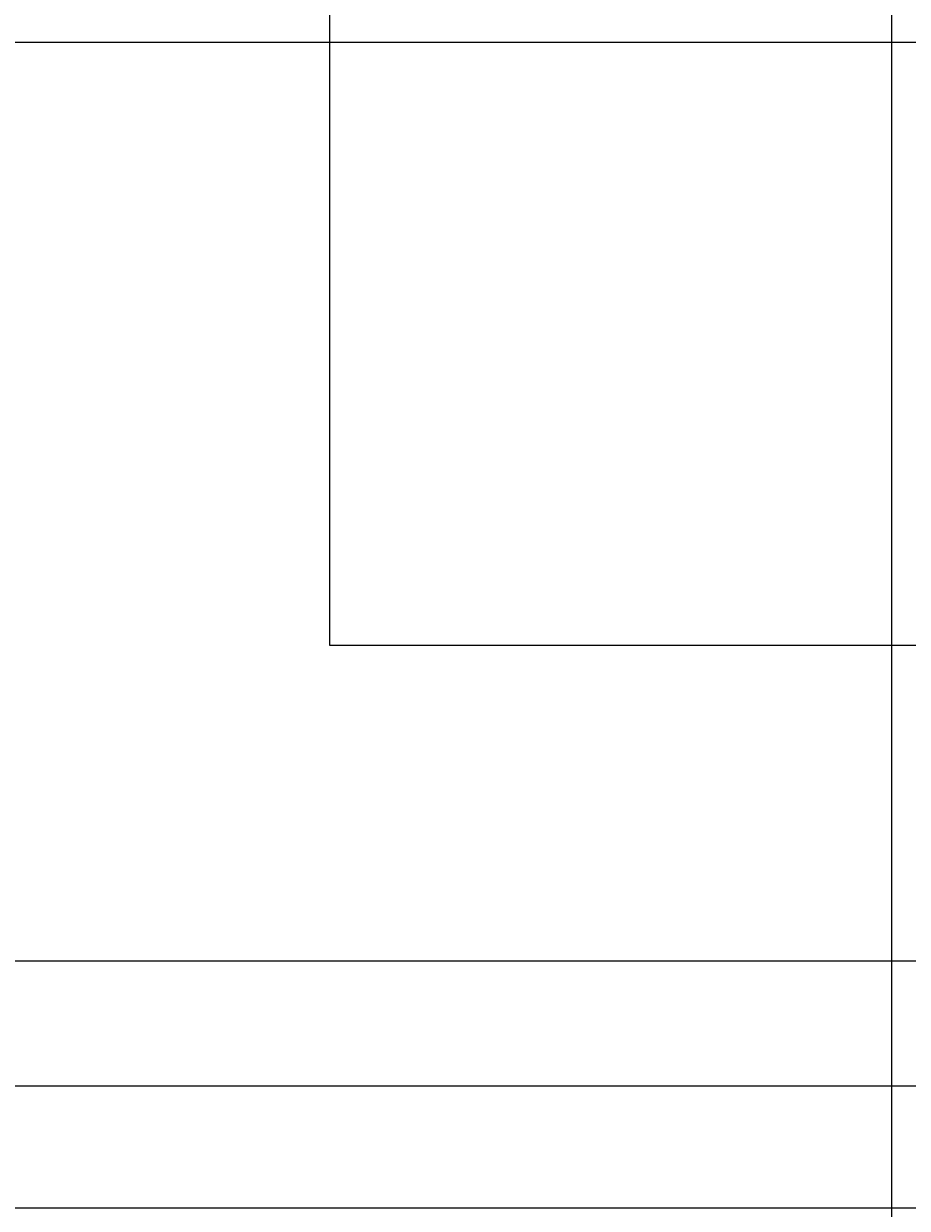
# Model space of a CAD drawing. Units: inches. Extents: x 35362 to 73946, y 43607 to 67532.
# Tile 87 of 134: x 51337 to 51924, y 47544 to 48331. Entities that reach past the tile are written whole.
import ezdxf

# ---------------------------------------------------------------- set-up
doc = ezdxf.new("R2010")
doc.units = ezdxf.units.IN
doc.header["$MEASUREMENT"] = 0
doc.layers.add('A-ANNO-DIMS', color=2, linetype='Continuous', lineweight=18)
doc.layers.add('E-WIRE', color=3, linetype='Continuous', lineweight=25)
doc.styles.get("Standard").update_dxf_attribs({"font": 'arial.ttf'})
doc.dimstyles.get("Standard").update_dxf_attribs({"dimtxt": 0.18, "dimasz": 0.18, "dimexe": 0.18, "dimexo": 0.0625, "dimgap": 0.09, "dimtad": 0, "dimtih": 1, "dimtoh": 1, "dimdec": 4, "dimzin": 0, "dimdsep": 46, "dimtxsty": 'Standard', "dimcen": 0.09, "dimadec": 0, "dimazin": 0, "dimtfac": 1, "dimtdec": 4, "dimtofl": 0, "dimtmove": 0, "dimatfit": 3, "dimfxl": 1, "dimtolj": 1, "dimtzin": 0, "dimarcsym": 0})

# ---------------------------------------------------------------- blocks, each defined once
blk = doc.blocks.new('*D11')
at = {"layer": 'A-ANNO-DIMS', "color": 0, "lineweight": -2, "transparency": 16777216}
for p, q in [((47978.66, 56028.77), (47978.66, 43606.68)), ((53109.76, 56028.77), (53109.76, 43606.68)), ((47978.84, 43606.86), (50543.87, 43606.86)), ((53109.58, 43606.86), (50544.55, 43606.86))]:
    blk.add_line(p, q, dxfattribs=at)
at = {"layer": 'A-ANNO-DIMS', "color": 0, "transparency": 16777216}
for points in [[(47978.84, 43606.89), (47978.84, 43606.83), (47978.66, 43606.86)], [(53109.58, 43606.89), (53109.58, 43606.83), (53109.76, 43606.86)]]:
    blk.add_solid(points, dxfattribs=at)
at = {"layer": 'Defpoints', "color": 0, "transparency": 16777216}
for p in [(47978.66, 56028.84), (53109.76, 56028.84), (53109.76, 43606.86)]:
    blk.add_point(p, dxfattribs=at)
at = {"layer": 'A-ANNO-DIMS', "color": 0, "transparency": 16777216, "insert": (50544.21, 43606.86), "char_height": 0.18, "attachment_point": 5}
blk.add_mtext('\\A1;5131', dxfattribs=at)
blk = doc.blocks.new('*D17')
at = {"layer": 'A-ANNO-DIMS', "color": 0, "lineweight": -2, "transparency": 16777216}
for p, q in [((49923.31, 61293.22), (49923.31, 43606.68)), ((51913.93, 61293.22), (51913.93, 43606.68)), ((49923.49, 43606.86), (50918.16, 43606.86)), ((51913.75, 43606.86), (50919.07, 43606.86))]:
    blk.add_line(p, q, dxfattribs=at)
at = {"layer": 'A-ANNO-DIMS', "color": 0, "transparency": 16777216}
for points in [[(49923.49, 43606.89), (49923.49, 43606.83), (49923.31, 43606.86)], [(51913.75, 43606.89), (51913.75, 43606.83), (51913.93, 43606.86)]]:
    blk.add_solid(points, dxfattribs=at)
at = {"layer": 'Defpoints', "color": 0, "transparency": 16777216}
for p in [(49923.31, 61293.29), (51913.93, 61293.29), (51913.93, 43606.86)]:
    blk.add_point(p, dxfattribs=at)
at = {"layer": 'A-ANNO-DIMS', "color": 0, "transparency": 16777216, "insert": (50918.62, 43606.86), "char_height": 0.18, "attachment_point": 5}
blk.add_mtext('\\A1;1990.6', dxfattribs=at)
blk = doc.blocks.new('*D43')
at = {"layer": 'A-ANNO-DIMS', "color": 0, "lineweight": -2, "transparency": 16777216}
for p, q in [((62004.67, 47625.18), (35361.77, 47625.18)), ((35361.95, 47625), (35361.95, 47416.9)), ((35361.95, 47208.43), (35361.95, 47416.53)), ((62004.67, 47208.25), (35361.77, 47208.25))]:
    blk.add_line(p, q, dxfattribs=at)
at = {"layer": 'A-ANNO-DIMS', "color": 0, "transparency": 16777216}
for points in [[(35361.92, 47625), (35361.98, 47625), (35361.95, 47625.18)], [(35361.92, 47208.43), (35361.98, 47208.43), (35361.95, 47208.25)]]:
    blk.add_solid(points, dxfattribs=at)
at = {"layer": 'Defpoints', "color": 0, "transparency": 16777216}
for p in [(62004.73, 47625.18), (35361.95, 47208.25), (62004.73, 47208.25)]:
    blk.add_point(p, dxfattribs=at)
at = {"layer": 'A-ANNO-DIMS', "color": 0, "transparency": 16777216, "insert": (35361.95, 47416.72), "char_height": 0.18, "attachment_point": 5}
blk.add_mtext('\\A1;416.9', dxfattribs=at)
blk = doc.blocks.new('*D67')
at = {"layer": 'A-ANNO-DIMS', "color": 0, "lineweight": -2, "transparency": 16777216}
for p, q in [((56873.54, 53351.53), (35361.77, 53351.53)), ((35361.95, 53351.35), (35361.95, 49400.89)), ((35361.95, 45450.07), (35361.95, 49400.53)), ((53793.58, 45449.89), (35361.77, 45449.89))]:
    blk.add_line(p, q, dxfattribs=at)
at = {"layer": 'A-ANNO-DIMS', "color": 0, "transparency": 16777216}
for points in [[(35361.92, 53351.35), (35361.98, 53351.35), (35361.95, 53351.53)], [(35361.92, 45450.07), (35361.98, 45450.07), (35361.95, 45449.89)]]:
    blk.add_solid(points, dxfattribs=at)
at = {"layer": 'Defpoints', "color": 0, "transparency": 16777216}
for p in [(35361.95, 53351.53), (56873.6, 53351.53), (53793.64, 45449.89)]:
    blk.add_point(p, dxfattribs=at)
at = {"layer": 'A-ANNO-DIMS', "color": 0, "transparency": 16777216, "insert": (35361.95, 49400.71), "char_height": 0.18, "attachment_point": 5}
blk.add_mtext('\\A1;7901.6', dxfattribs=at)
blk = doc.blocks.new('*D87')
at = {"layer": 'A-ANNO-DIMS', "color": 0, "lineweight": -2, "transparency": 16777216}
for p, q in [((52362.49, 48318.27), (35361.77, 48318.27)), ((35361.95, 48318.09), (35361.95, 47931.38)), ((35361.95, 47544.31), (35361.95, 47931.02)), ((52362.49, 47544.13), (35361.77, 47544.13))]:
    blk.add_line(p, q, dxfattribs=at)
at = {"layer": 'A-ANNO-DIMS', "color": 0, "transparency": 16777216}
for points in [[(35361.92, 48318.09), (35361.98, 48318.09), (35361.95, 48318.27)], [(35361.92, 47544.31), (35361.98, 47544.31), (35361.95, 47544.13)]]:
    blk.add_solid(points, dxfattribs=at)
at = {"layer": 'Defpoints', "color": 0, "transparency": 16777216}
for p in [(35361.95, 48318.27), (52362.56, 48318.27), (52362.56, 47544.13)]:
    blk.add_point(p, dxfattribs=at)
at = {"layer": 'A-ANNO-DIMS', "color": 0, "transparency": 16777216, "insert": (35361.95, 47931.2), "char_height": 0.18, "attachment_point": 5}
blk.add_mtext('\\A1;774.1', dxfattribs=at)
blk = doc.blocks.new('*D89')
at = {"layer": 'A-ANNO-DIMS', "color": 0, "lineweight": -2, "transparency": 16777216}
for p, q in [((53707.72, 48897.74), (35361.77, 48897.74)), ((35361.95, 48897.56), (35361.95, 48303.16)), ((35361.95, 47708.4), (35361.95, 48302.8)), ((53707.72, 47708.22), (35361.77, 47708.22))]:
    blk.add_line(p, q, dxfattribs=at)
at = {"layer": 'A-ANNO-DIMS', "color": 0, "transparency": 16777216}
for points in [[(35361.92, 48897.56), (35361.98, 48897.56), (35361.95, 48897.74)], [(35361.92, 47708.4), (35361.98, 47708.4), (35361.95, 47708.22)]]:
    blk.add_solid(points, dxfattribs=at)
at = {"layer": 'Defpoints', "color": 0, "transparency": 16777216}
for p in [(53707.78, 48897.74), (35361.95, 47708.22), (53707.78, 47708.22)]:
    blk.add_point(p, dxfattribs=at)
at = {"layer": 'A-ANNO-DIMS', "color": 0, "transparency": 16777216, "insert": (35361.95, 48302.98), "char_height": 0.18, "attachment_point": 5}
blk.add_mtext('\\A1;1189.5', dxfattribs=at)

msp = doc.modelspace()

# ---------------------------------------------------------------- linework, layer by layer
at = {"layer": 'E-WIRE'}
for p, q in [((51540.551, 48956.924), (51540.551, 47918.089)), ((51540.551, 47918.089), (52061.002, 47918.089))]:
    msp.add_line(p, q, dxfattribs=at)

# ---------------------------------------------------------------- dimensions: what is measured, and where the dimension line sits
at = {"layer": 'A-ANNO-DIMS'}
for base, p1, p2, override, picture, middle in [((51913.931, 43606.859), (49923.307, 61293.286), (51913.931, 61293.286), {"dimdec": 1, "dimlfac": 1, "dimrnd": 0, "dimzin": 0, "dimdsep": 46, "dimlunit": 2}, '*D17', (50918.619, 43606.859)), ((53109.76, 43606.859), (47978.665, 56028.836), (53109.76, 56028.836), {"dimdec": 0, "dimlfac": 1, "dimrnd": 0, "dimzin": 0, "dimdsep": 46, "dimlunit": 2}, '*D11', (50544.212, 43606.859))]:
    dim = msp.add_linear_dim(base=base, p1=p1, p2=p2, dimstyle='Standard', override=override, dxfattribs=at)
    dim.commit()
    dim.dimension.update_dxf_attribs({"geometry": picture, "text_midpoint": middle})
for base, p1, p2, picture, middle in [((35361.949, 53351.529), (53793.638, 45449.894), (56873.602, 53351.529), '*D67', (35361.949, 49400.712)), ((35361.949, 47708.216), (53707.781, 48897.738), (53707.781, 47708.216), '*D89', (35361.949, 48302.977)), ((35361.949, 48318.269), (52362.557, 47544.134), (52362.557, 48318.269), '*D87', (35361.949, 47931.201)), ((35361.949, 47208.25), (62004.728, 47625.181), (62004.728, 47208.25), '*D43', (35361.949, 47416.715))]:
    dim = msp.add_linear_dim(base=base, p1=p1, p2=p2, angle=90, dimstyle='Standard', override={"dimdec": 1, "dimlfac": 1, "dimrnd": 0, "dimzin": 0, "dimdsep": 46, "dimlunit": 2}, dxfattribs=at)
    dim.commit()
    dim.dimension.update_dxf_attribs({"geometry": picture, "text_midpoint": middle})

doc.saveas('drawing.dxf')
